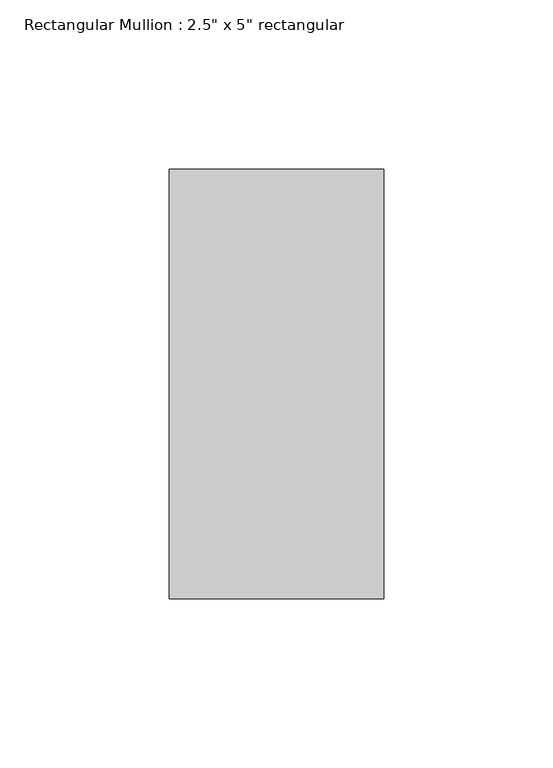
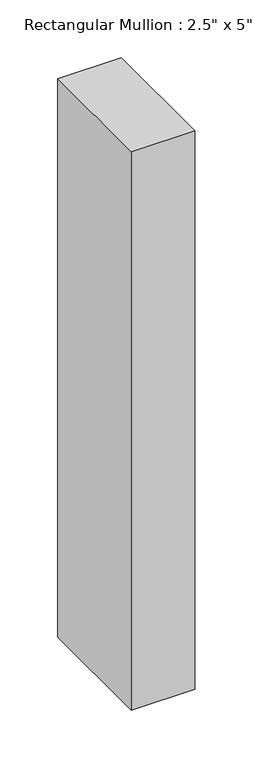
"""IFC4 building model written with IfcOpenShell, lengths in millimetres: member geometry."""

from ifc_helpers import new_model, si_unit, frame, origin, place, context, project, spatial, polyline, outline, extrude, source, transform, mapped, element, save


def member_501b078b(model_context):
    return source(origin(), model_context, "Body", "SweptSolid", [
        extrude(outline(polyline([(0.0, 63.5), (0.0, -63.5), (-63.5, -63.5), (-63.5, 63.5), (0.0, 63.5)])), frame((0.0, 0.0, -589.425288), z_axis=(0.0, 0.0, 1.0), x_axis=(1.0, 0.0, 0.0)), (0.0, 0.0, 1.0), 589.425288),
    ])


if __name__ == "__main__":
    model = new_model("IFC4")
    model_context = context("Model", 3, world=origin())
    ifc_project = project(units=[si_unit("LENGTHUNIT", "METRE", prefix="MILLI")], contexts=[model_context])
    site = spatial("IfcSite", under=ifc_project)
    building = spatial("IfcBuilding", under=site)
    placement = place(None, origin())
    member_shape = member_501b078b(model_context)
    element("IfcMember", 1, ObjectType="Rectangular Mullion : 2.5\" x 5\" rectangular", at=placement, inside=building, context=model_context, shape_type="MappedRepresentation", body=[
        mapped(member_shape, transform((0.0, 0.0, 0.0), x_axis=(1.0, 0.0, 0.0), y_axis=(0.0, 1.0, 0.0), z_axis=(0.0, 0.0, 1.0))),
    ])
    save(model, "model.ifc")

# Revit data of these elements
# Type "Rectangular Mullion : 2.5\" x 5\" rectangular"
#   built-in parameter 1007304 = 0.416667 (stored number, unit not read)
#   built-in parameter 1007301 = 0.104167 (stored number, unit not read)
#   built-in parameter 1007300 = 0.104167 (stored number, unit not read)
# Element 1 (IfcMember, "Rectangular Mullion : 2.5\" x 5\" rectangular")
#   Materials on its faces: "Aluminum"
# Materials
#   "Aluminum": class "Metal", colour RGB 247 247 247, transparency 0, Description = "Aluminum 6061", Cost = 0
